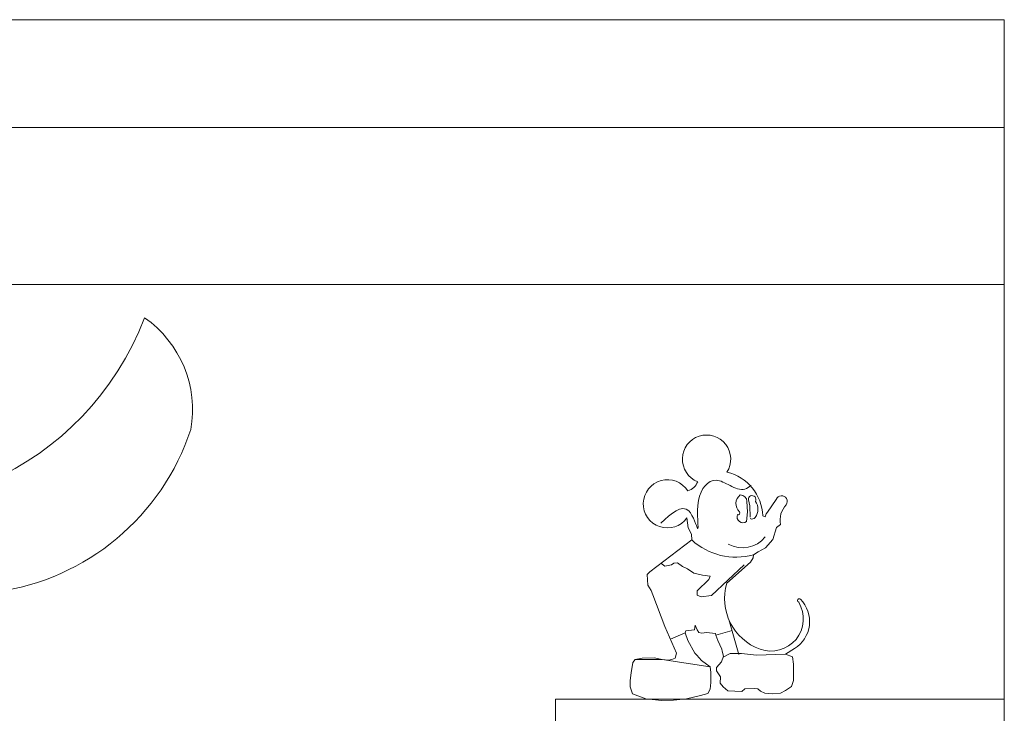
# Model space of a CAD drawing. Units: inches. Extents: x -17 to 1735, y -531 to 60.
# Tile 26 of 27: x 1734.79189 to 1734.82789, y -150.18755 to -150.1622. Entities that reach past the tile are written whole.
import ezdxf

# ---------------------------------------------------------------- set-up
doc = ezdxf.new("R2010")
doc.units = ezdxf.units.IN
doc.header["$MEASUREMENT"] = 0
doc.layers.add('A-FURN', color=242, linetype='Continuous', lineweight=18, true_color=0xcd2027)

# ---------------------------------------------------------------- blocks, each defined once
blk = doc.blocks.new('childrens_room_2')
for p, q in [((72.04826, 55.53364), (74.04826, 55.53364)), ((74.04826, 55.53364), (74.04826, 52.93364)), ((72.04826, 55.43364), (74.04826, 55.43364)), ((72.04826, 55.28795), (74.04826, 55.28795)), ((73.79248, 54.97681), (73.80175, 54.94446)), ((73.75195, 54.96452), (73.73816, 54.9585)), ((73.78052, 54.96237), (73.7954, 54.96663)), ((73.70556, 54.93988), (73.73062, 54.93968)), ((73.73062, 54.93968), (73.77504, 54.93304)), ((73.63163, 54.17766), (73.63163, 54.90289)), ((74.04826, 54.90289), (73.63163, 54.90289))]:
    blk.add_line(p, q)
for points in [[(73.79073, 55.11362, 2.780632), (73.76353, 55.10482, -0.231731), (73.75433, 55.09622, 3.269279), (73.75355, 55.07118), (73.75471, 55.06209), (73.75764, 55.05622), (73.75803, 55.05075), (73.71909, 55.02102), (73.71674, 55.01868), (73.71732, 55.0087), (73.72026, 55.00381), (73.72202, 54.99971), (73.73296, 54.97039), (73.74373, 54.94575), (73.74255, 54.94086), (73.73962, 54.93968), (73.7361, 54.93929), (73.73062, 54.93968), (73.72298, 54.94125), (73.71202, 54.94105), (73.70556, 54.93988), (73.70341, 54.93695), (73.70263, 54.93304), (73.70185, 54.92756), (73.70087, 54.91993), (73.70087, 54.91426), (73.70302, 54.908), (73.71535, 54.90331), (73.73022, 54.90175), (73.74099, 54.90194), (73.75312, 54.90311), (73.76624, 54.90644), (73.77309, 54.9082), (73.77524, 54.91211), (73.77583, 54.91837), (73.77583, 54.92756), (73.77504, 54.93304), (73.76721, 54.93871), (73.76271, 54.94379), (73.76095, 54.94575), (73.7543, 54.95729), (73.75195, 54.96452), (73.75254, 54.96628), (73.76056, 54.96726), (73.76115, 54.97176), (73.7631, 54.96745), (73.76447, 54.96491), (73.76741, 54.96433), (73.77172, 54.96472), (73.77994, 54.96393), (73.78052, 54.96237), (73.78228, 54.95729), (73.786, 54.94927), (73.78639, 54.94751), (73.78737, 54.94281), (73.78561, 54.93753), (73.78111, 54.93245), (73.78091, 54.92932), (73.78209, 54.92736), (73.78463, 54.92365), (73.78444, 54.91778), (73.78718, 54.91426), (73.79139, 54.91069), (73.79804, 54.9103), (73.8045, 54.90991), (73.80724, 54.91265), (73.81644, 54.91284), (73.81937, 54.91265), (73.82192, 54.9105), (73.82603, 54.90854), (73.83268, 54.90796), (73.84032, 54.90854), (73.84521, 54.91089), (73.85069, 54.9148), (73.85245, 54.92028), (73.85265, 54.92829), (73.85265, 54.93553), (73.85147, 54.94237), (73.84501, 54.94472), (73.85343, 54.9499, 0.480393), (73.8591, 54.99566, 1.257082), (73.85734, 54.99292, -0.706408), (73.82152, 54.94931, -0.397958), (73.7906, 55.01072), (73.81272, 55.03), (73.81507, 55.0341), (73.81526, 55.03704), (73.81957, 55.03978), (73.82642, 55.0433), (73.83346, 55.05112), (73.8366, 55.06226), (73.84046, 55.06496)], [(73.82836, 55.07647), (73.82713, 55.07486), (73.82615, 55.07212), (73.82399, 55.0731, 0.337972), (73.79073, 55.11362)], [(73.8089, 55.06779), (73.80975, 55.07676), (73.80931, 55.08637, 0.410066), (73.80288, 55.09246, 0.451179), (73.8023, 55.07693, -0.84041), (73.80044, 55.07422, 0.740597), (73.8089, 55.06779)], [(73.81242, 55.0718), (73.81208, 55.08246), (73.81079, 55.08801, -0.357136), (73.81266, 55.09157, -0.713549), (73.81723, 55.08649, -0.314811), (73.81706, 55.0716, -0.383013), (73.81225, 55.07061, 0.242652)], [(73.82836, 55.07647), (73.83654, 55.0884, -1.147535), (73.84572, 55.08345, 0.239038), (73.84046, 55.06496, -0.932314)]]:
    blk.add_lwpolyline(points, format="xyb")
for points in [[(73.80667, 55.02778), (73.77649, 54.99925), (73.76676, 54.99795), (73.76319, 54.99957), (73.76319, 55.00346), (73.7739, 55.01416), (73.7752, 55.01708), (73.76806, 55.01805), (73.75995, 55.02), (73.75411, 55.02389), (73.74957, 55.02616), (73.7447, 55.0294), (73.74145, 55.02908), (73.73918, 55.02778), (73.73302, 55.02648), (73.72945, 55.02908)], [(73.84501, 54.94472), (73.81803, 54.94364), (73.80419, 54.94527), (73.79361, 54.94527), (73.7871, 54.94202)]]:
    blk.add_lwpolyline(points)
for centre, radius, start, end in [((72.9941, 55.35488), 0.27385, 249.35307, 339.06179), ((73.19055, 55.17174), 0.10388, 349.70856, 55.1818), ((73.08182, 55.22246), 0.22203, 213.90153, 341.8175), ((73.7989, 55.09502), 0.06025, 227.29331, 285.75945), ((73.80523, 55.07004), 0.02665, 240.06884, 321.89185)]:
    blk.add_arc(centre, radius, start, end)
blk.add_open_spline([(73.81311, 55.10124), (73.81125, 55.09991), (73.80537, 55.0957), (73.79345, 55.10101), (73.77697, 55.11046), (73.75935, 55.09095), (73.76677, 55.04784), (73.75493, 55.08994), (73.739, 55.07524), (73.72929, 55.06627)], degree=3, knots=[0, 0, 0, 0, 0.0065598, 0.0207717, 0.0346767, 0.0594701, 0.0855043, 0.1036903, 0.1321117, 0.1321117, 0.1321117, 0.1321117])

msp = doc.modelspace()

# ---------------------------------------------------------------- block references
at = {"layer": 'A-FURN', "xscale": 0.0393700787401575, "yscale": 0.0393700787401575, "zscale": 0.0393700787401575}
msp.add_blockref('childrens_room_2', (1731.912601, -152.348565), dxfattribs=at)

doc.saveas('drawing.dxf')
